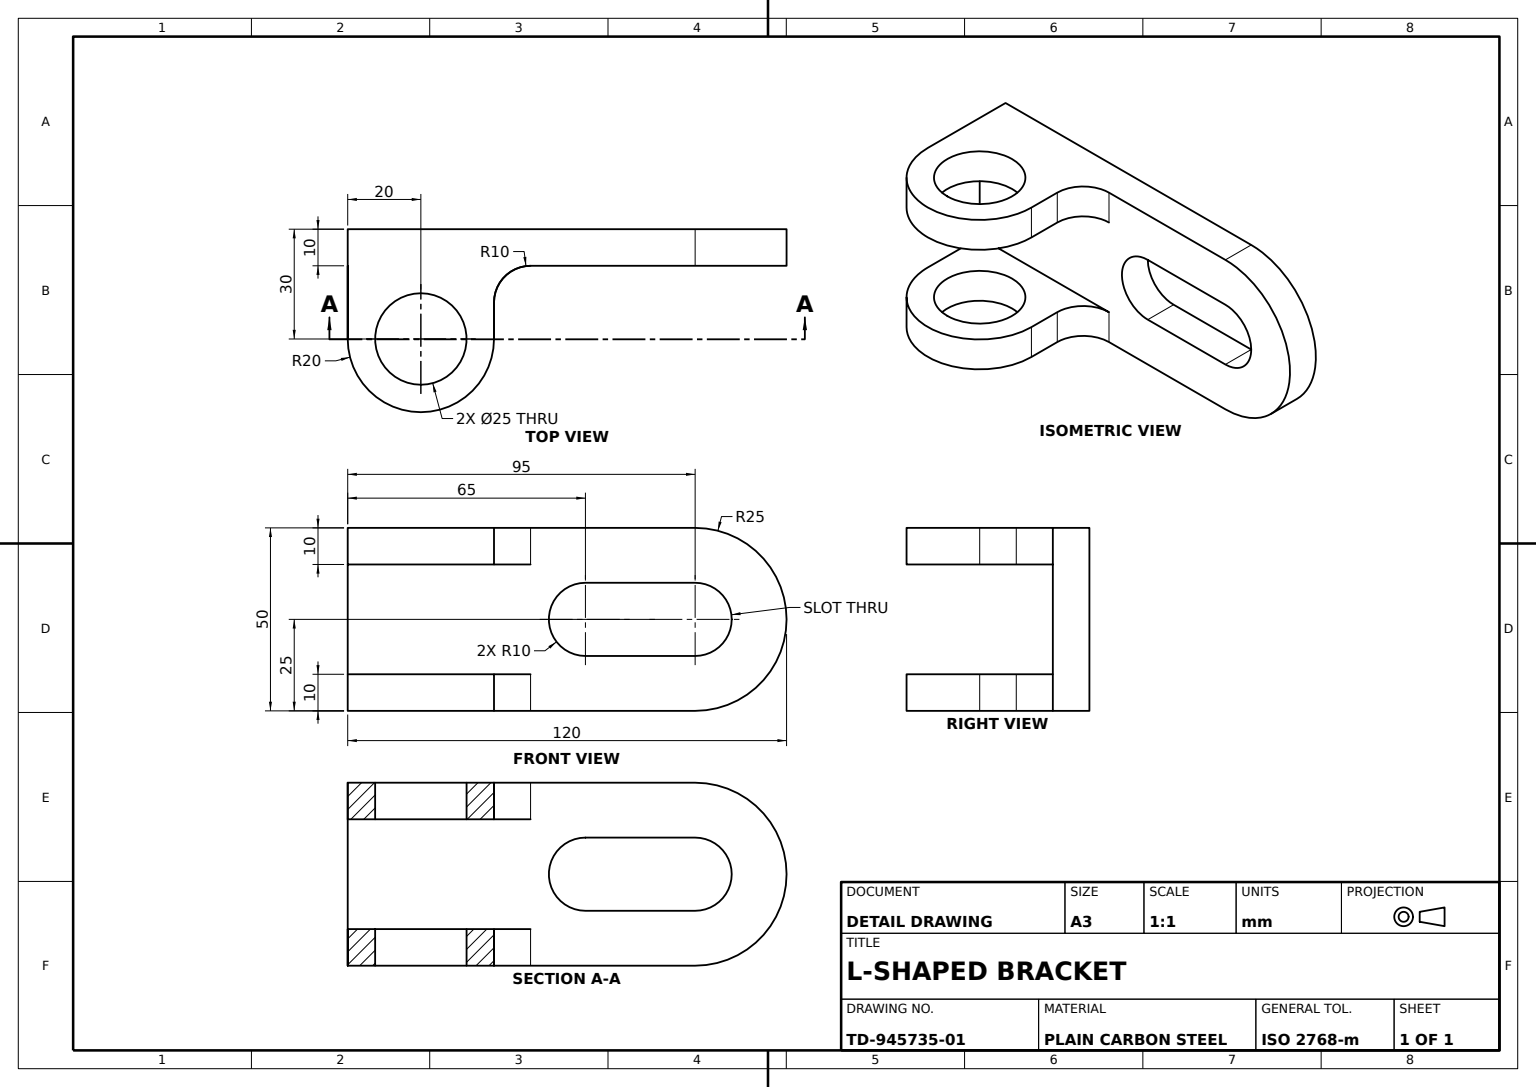
from build123d import *

# Parameters (mm, degrees)
BASE_PLATE_DEPTH  = 10
SLOT_CUT_DEPTH    = 10
LUG_1_DEPTH       = 10
LUG_START         = -10
LUG_2_DEPTH       = 10
PIN_HOLE_SKETCH_R = 12.5
PIN_HOLE_25_DEPTH = 50


with BuildPart() as part:
    # Base Plate Sketch → Base Plate (new body)
    with BuildSketch(Plane.XY):
        with BuildLine():
            Line((95, 25), (0, 25))
            Line((0, 25), (0, -25))
            Line((0, -25), (95, -25))
            ThreePointArc((95, -25), (120, 0), (95, 25))
        make_face()
    extrude(amount=BASE_PLATE_DEPTH)

    # Slot Sketch → Slot Cut (cut)
    with BuildSketch(Plane.XY.offset(10)):
        with BuildLine():
            Line((65, 10), (95, 10))
            ThreePointArc((95, 10), (105, 0), (95, -10))
            Line((95, -10), (65, -10))
            ThreePointArc((65, -10), (55, 0), (65, 10))
        make_face()
    extrude(amount=-SLOT_CUT_DEPTH, mode=Mode.SUBTRACT)

    # Lug 1 Sketch → Lug 1 (add)
    with BuildSketch(Plane.XZ.offset(25)):
        with BuildLine():
            Line((0, 10), (0, 30))
            ThreePointArc((0, 30), (20, 50), (40, 30))
            Line((40, 30), (40, 20))
            ThreePointArc((40, 20), (42.928932188, 12.928932188), (50, 10))
            Line((50, 10), (0, 10))
        make_face()
    extrude(amount=-LUG_1_DEPTH)

    # Lug 2 Sketch → Lug 2 (add)
    with BuildSketch(Plane(origin=(0, 25, 0), x_dir=(1, 0, 0), z_dir=(0, 1, 0)).offset(LUG_START)):
        with BuildLine():
            Line((0, -30), (0, -10))
            Line((0, -10), (50, -10))
            ThreePointArc((50, -10), (42.928932188, -12.928932188), (40, -20))
            Line((40, -20), (40, -30))
            ThreePointArc((40, -30), (20, -50), (0, -30))
        make_face()
    extrude(amount=LUG_2_DEPTH)

    # Pin Hole Sketch → Pin Hole Ø25 (cut)
    with BuildSketch(Plane.XZ.offset(25)):
        with Locations(Location((20, 30, 0), (0, 0, 270))):
            Circle(PIN_HOLE_SKETCH_R)
    extrude(amount=-PIN_HOLE_25_DEPTH, mode=Mode.SUBTRACT)


solid = part.part
